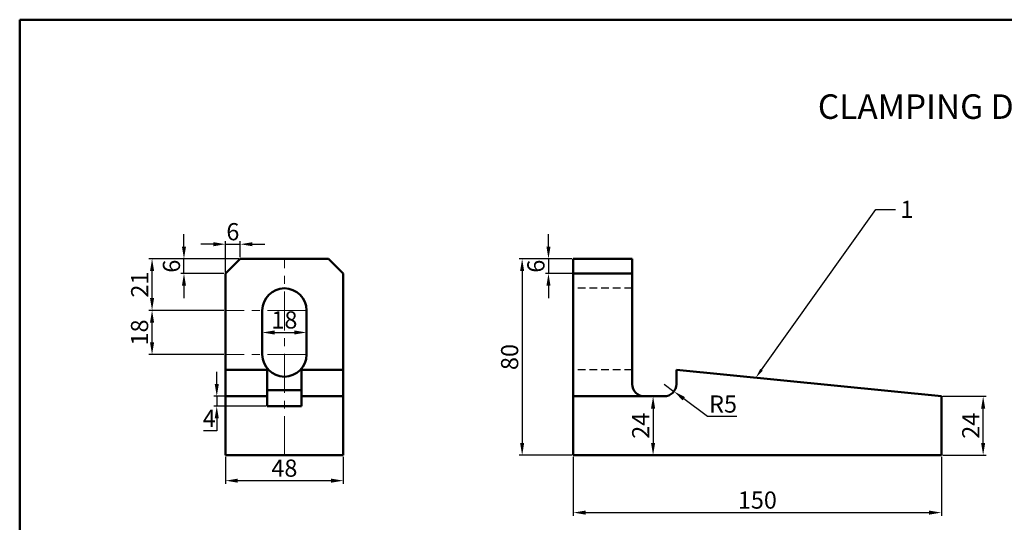
# Model space of a CAD drawing. Units: millimetres. Extents: x -238 to 500, y -191 to 322.
# Tile 2 of 3: x -238 to 164, y 117 to 322. Entities that reach past the tile are written whole.
import ezdxf
from ezdxf import colors
from ezdxf.entities.mleader import LeaderData, LeaderLine
from ezdxf.math import Vec2, Vec3

# ---------------------------------------------------------------- set-up
doc = ezdxf.new("R2010")
doc.units = ezdxf.units.MM
doc.header["$LTSCALE"] = 0.5
doc.linetypes.add('CENTER', pattern=[50.8, 31.75, -6.35, 6.35, -6.35])
doc.linetypes.add('DASHED', pattern=[19.05, 12.7, -6.35])
for name, color, linetype, lineweight in [('M-CNTR', 1, 'CENTER', 18), ('M-DIMS', 2, 'Continuous', 25), ('M-HIDN', 6, 'DASHED', 25), ('M-OUTL', 7, 'Continuous', 50), ('M-TEXT', 3, 'Continuous', 25), ('M-TTLB', 7, 'Continuous', 50)]:
    doc.layers.add(name, color=color, linetype=linetype, lineweight=lineweight)
doc.styles.get("Standard").update_dxf_attribs({"font": 'arial.ttf'})
doc.dimstyles.new('ISO-25', dxfattribs={"dimtxt": 7, "dimasz": 5, "dimexe": 1.25, "dimexo": 0.625, "dimtad": 1, "dimtoh": 1, "dimtxsty": 'Standard', "dimcen": 2.5, "dimadec": 0, "dimazin": 0, "dimtfac": 1, "dimtmove": 0, "dimatfit": 3, "dimfxl": 1, "dimarcsym": 0})

# ---------------------------------------------------------------- blocks, each defined once
blk = doc.blocks.new('*D5')
at = {"layer": 'Defpoints', "color": 0, "ltscale": 0.5, "transparency": 16777216}
for p in [(-12.02, 144.24), (137.98, 144.24), (137.98, 120.87)]:
    blk.add_point(p, dxfattribs=at)
at = {"layer": 'M-DIMS', "color": 0, "lineweight": -2, "ltscale": 0.5, "transparency": 16777216}
for p, q in [((-12.02, 143.61), (-12.02, 119.62)), ((137.98, 143.61), (137.98, 119.62)), ((-7.02, 120.87), (132.98, 120.87))]:
    blk.add_line(p, q, dxfattribs=at)
at = {"layer": 'M-DIMS', "color": 0, "ltscale": 0.5, "transparency": 16777216}
for points in [[(-7.02, 121.7), (-7.02, 120.04), (-12.02, 120.87)], [(132.98, 121.7), (132.98, 120.04), (137.98, 120.87)]]:
    blk.add_solid(points, dxfattribs=at)
at = {"layer": 'M-DIMS', "color": 0, "ltscale": 0.5, "transparency": 16777216, "insert": (62.98, 125.07), "char_height": 7, "attachment_point": 5}
blk.add_mtext('150', dxfattribs=at)
blk = doc.blocks.new('*D6')
at = {"layer": 'Defpoints', "color": 0, "ltscale": 0.5, "transparency": 16777216}
for p in [(-12.02, 224.24), (-32.87, 144.24), (-12.02, 144.24)]:
    blk.add_point(p, dxfattribs=at)
at = {"layer": 'M-DIMS', "color": 0, "lineweight": -2, "ltscale": 0.5, "transparency": 16777216}
for p, q in [((-12.65, 224.24), (-34.12, 224.24)), ((-32.87, 219.24), (-32.87, 149.24)), ((-12.65, 144.24), (-34.12, 144.24))]:
    blk.add_line(p, q, dxfattribs=at)
at = {"layer": 'M-DIMS', "color": 0, "ltscale": 0.5, "transparency": 16777216}
for points in [[(-33.71, 219.24), (-32.04, 219.24), (-32.87, 224.24)], [(-33.71, 149.24), (-32.04, 149.24), (-32.87, 144.24)]]:
    blk.add_solid(points, dxfattribs=at)
at = {"layer": 'M-DIMS', "color": 0, "ltscale": 0.5, "transparency": 16777216, "insert": (-37.07, 184.24), "char_height": 7, "attachment_point": 5, "rotation": 90}
blk.add_mtext('80', dxfattribs=at)
blk = doc.blocks.new('*D7')
at = {"layer": 'Defpoints', "color": 0, "ltscale": 0.5, "transparency": 16777216}
for p in [(-12.02, 224.24), (-22.15, 218.24), (-12.02, 218.24)]:
    blk.add_point(p, dxfattribs=at)
at = {"layer": 'M-DIMS', "color": 0, "lineweight": -2, "ltscale": 0.5, "transparency": 16777216}
for p, q in [((-22.15, 229.24), (-22.15, 234.24)), ((-12.65, 224.24), (-23.4, 224.24)), ((-22.15, 224.24), (-22.15, 218.24)), ((-12.65, 218.24), (-23.4, 218.24)), ((-22.15, 213.24), (-22.15, 208.24))]:
    blk.add_line(p, q, dxfattribs=at)
at = {"layer": 'M-DIMS', "color": 0, "ltscale": 0.5, "transparency": 16777216}
for points in [[(-22.99, 229.24), (-21.32, 229.24), (-22.15, 224.24)], [(-22.99, 213.24), (-21.32, 213.24), (-22.15, 218.24)]]:
    blk.add_solid(points, dxfattribs=at)
at = {"layer": 'M-DIMS', "color": 0, "ltscale": 0.5, "transparency": 16777216, "insert": (-26.35, 221.24), "char_height": 7, "attachment_point": 5, "rotation": 90}
blk.add_mtext('6', dxfattribs=at)
blk = doc.blocks.new('*D8')
at = {"layer": 'Defpoints', "color": 0, "ltscale": 0.5, "transparency": 16777216}
for p in [(137.98, 168.24), (155, 168.24), (137.98, 144.24)]:
    blk.add_point(p, dxfattribs=at)
at = {"layer": 'M-DIMS', "color": 0, "lineweight": -2, "ltscale": 0.5, "transparency": 16777216}
for p, q in [((138.6, 168.24), (156.25, 168.24)), ((155, 149.24), (155, 163.24)), ((138.6, 144.24), (156.25, 144.24))]:
    blk.add_line(p, q, dxfattribs=at)
at = {"layer": 'M-DIMS', "color": 0, "ltscale": 0.5, "transparency": 16777216}
for points in [[(154.16, 163.24), (155.83, 163.24), (155, 168.24)], [(154.16, 149.24), (155.83, 149.24), (155, 144.24)]]:
    blk.add_solid(points, dxfattribs=at)
at = {"layer": 'M-DIMS', "color": 0, "ltscale": 0.5, "transparency": 16777216, "insert": (150.86, 156.24), "char_height": 7, "attachment_point": 5, "rotation": 90}
blk.add_mtext('24', dxfattribs=at)
blk = doc.blocks.new('*D9')
at = {"layer": 'Defpoints', "color": 0, "ltscale": 0.5, "transparency": 16777216}
for p in [(20.98, 168.24), (20.49, 144.24), (20.98, 144.24)]:
    blk.add_point(p, dxfattribs=at)
at = {"layer": 'M-DIMS', "color": 0, "lineweight": -2, "ltscale": 0.5, "transparency": 16777216}
for p, q in [((20.35, 168.24), (19.24, 168.24)), ((20.49, 163.24), (20.49, 149.24)), ((20.35, 144.24), (19.24, 144.24))]:
    blk.add_line(p, q, dxfattribs=at)
at = {"layer": 'M-DIMS', "color": 0, "ltscale": 0.5, "transparency": 16777216}
for points in [[(19.65, 163.24), (21.32, 163.24), (20.49, 168.24)], [(19.65, 149.24), (21.32, 149.24), (20.49, 144.24)]]:
    blk.add_solid(points, dxfattribs=at)
at = {"layer": 'M-DIMS', "color": 0, "ltscale": 0.5, "transparency": 16777216, "insert": (16.35, 156.24), "char_height": 7, "attachment_point": 5, "rotation": 90}
blk.add_mtext('24', dxfattribs=at)
blk = doc.blocks.new('*D10')
at = {"layer": 'Defpoints', "color": 0, "ltscale": 0.5, "transparency": 16777216}
for p in [(24.98, 173.24), (28.98, 170.25)]:
    blk.add_point(p, dxfattribs=at)
at = {"layer": 'M-DIMS', "color": 0, "lineweight": -2, "ltscale": 0.5, "transparency": 16777216}
for p, q in [((24.98, 173.24), (28.98, 170.25)), ((42.7, 160.01), (32.99, 167.26)), ((54.67, 160.01), (42.7, 160.01))]:
    blk.add_line(p, q, dxfattribs=at)
at = {"layer": 'M-DIMS', "color": 0, "ltscale": 0.5, "transparency": 16777216}
blk.add_solid([(33.49, 167.92), (32.49, 166.59), (28.98, 170.25)], dxfattribs=at)
at = {"layer": 'M-DIMS', "color": 0, "ltscale": 0.5, "transparency": 16777216, "insert": (49, 164.19), "char_height": 7, "attachment_point": 5}
blk.add_mtext('R5', dxfattribs=at)
blk = doc.blocks.new('*D11')
at = {"layer": 'Defpoints', "color": 0, "ltscale": 0.5, "transparency": 16777216}
for p in [(-147.77, 230.19), (-147.77, 224.24), (-153.77, 218.24)]:
    blk.add_point(p, dxfattribs=at)
at = {"layer": 'M-DIMS', "color": 0, "lineweight": -2, "ltscale": 0.5, "transparency": 16777216}
for p, q in [((-158.77, 230.19), (-163.77, 230.19)), ((-153.77, 218.86), (-153.77, 231.44)), ((-153.77, 230.19), (-147.77, 230.19)), ((-147.77, 224.86), (-147.77, 231.44)), ((-142.77, 230.19), (-137.77, 230.19))]:
    blk.add_line(p, q, dxfattribs=at)
at = {"layer": 'M-DIMS', "color": 0, "ltscale": 0.5, "transparency": 16777216}
for points in [[(-158.77, 231.02), (-158.77, 229.35), (-153.77, 230.19)], [(-142.77, 231.02), (-142.77, 229.35), (-147.77, 230.19)]]:
    blk.add_solid(points, dxfattribs=at)
at = {"layer": 'M-DIMS', "color": 0, "ltscale": 0.5, "transparency": 16777216, "insert": (-150.77, 234.38), "char_height": 7, "attachment_point": 5}
blk.add_mtext('6', dxfattribs=at)
blk = doc.blocks.new('*D12')
at = {"layer": 'Defpoints', "color": 0, "ltscale": 0.5, "transparency": 16777216}
for p in [(-170.69, 224.24), (-147.77, 224.24), (-153.77, 218.24)]:
    blk.add_point(p, dxfattribs=at)
at = {"layer": 'M-DIMS', "color": 0, "lineweight": -2, "ltscale": 0.5, "transparency": 16777216}
for p, q in [((-170.69, 229.24), (-170.69, 234.24)), ((-148.39, 224.24), (-171.94, 224.24)), ((-170.69, 218.24), (-170.69, 224.24)), ((-154.39, 218.24), (-171.94, 218.24)), ((-170.69, 213.24), (-170.69, 208.24))]:
    blk.add_line(p, q, dxfattribs=at)
at = {"layer": 'M-DIMS', "color": 0, "ltscale": 0.5, "transparency": 16777216}
for points in [[(-171.52, 229.24), (-169.85, 229.24), (-170.69, 224.24)], [(-171.52, 213.24), (-169.85, 213.24), (-170.69, 218.24)]]:
    blk.add_solid(points, dxfattribs=at)
at = {"layer": 'M-DIMS', "color": 0, "ltscale": 0.5, "transparency": 16777216, "insert": (-174.88, 221.24), "char_height": 7, "attachment_point": 5, "rotation": 90}
blk.add_mtext('6', dxfattribs=at)
blk = doc.blocks.new('*D13')
at = {"layer": 'Defpoints', "color": 0, "ltscale": 0.5, "transparency": 16777216}
for p in [(-183.7, 224.24), (-153.77, 224.24), (-153.77, 203.24)]:
    blk.add_point(p, dxfattribs=at)
at = {"layer": 'M-DIMS', "color": 0, "lineweight": -2, "ltscale": 0.5, "transparency": 16777216}
for p, q in [((-154.39, 224.24), (-184.95, 224.24)), ((-183.7, 208.24), (-183.7, 219.24)), ((-154.39, 203.24), (-184.95, 203.24))]:
    blk.add_line(p, q, dxfattribs=at)
at = {"layer": 'M-DIMS', "color": 0, "ltscale": 0.5, "transparency": 16777216}
for points in [[(-184.53, 219.24), (-182.86, 219.24), (-183.7, 224.24)], [(-184.53, 208.24), (-182.86, 208.24), (-183.7, 203.24)]]:
    blk.add_solid(points, dxfattribs=at)
at = {"layer": 'M-DIMS', "color": 0, "ltscale": 0.5, "transparency": 16777216, "insert": (-187.83, 213.74), "char_height": 7, "attachment_point": 5, "rotation": 90}
blk.add_mtext('21', dxfattribs=at)
blk = doc.blocks.new('*D14')
at = {"layer": 'Defpoints', "color": 0, "ltscale": 0.5, "transparency": 16777216}
for p in [(-183.7, 203.24), (-153.77, 203.24), (-153.77, 185.24)]:
    blk.add_point(p, dxfattribs=at)
at = {"layer": 'M-DIMS', "color": 0, "lineweight": -2, "ltscale": 0.5, "transparency": 16777216}
for p, q in [((-154.39, 203.24), (-184.95, 203.24)), ((-183.7, 190.24), (-183.7, 198.24)), ((-154.39, 185.24), (-184.95, 185.24))]:
    blk.add_line(p, q, dxfattribs=at)
at = {"layer": 'M-DIMS', "color": 0, "ltscale": 0.5, "transparency": 16777216}
for points in [[(-184.53, 198.24), (-182.86, 198.24), (-183.7, 203.24)], [(-184.53, 190.24), (-182.86, 190.24), (-183.7, 185.24)]]:
    blk.add_solid(points, dxfattribs=at)
at = {"layer": 'M-DIMS', "color": 0, "ltscale": 0.5, "transparency": 16777216, "insert": (-187.89, 194.24), "char_height": 7, "attachment_point": 5, "rotation": 90}
blk.add_mtext('18', dxfattribs=at)
blk = doc.blocks.new('*D15')
at = {"layer": 'Defpoints', "color": 0, "ltscale": 0.5, "transparency": 16777216}
for p in [(-136.77, 168.24), (-157.33, 164.24), (-136.77, 164.24)]:
    blk.add_point(p, dxfattribs=at)
at = {"layer": 'M-DIMS', "color": 0, "lineweight": -2, "ltscale": 0.5, "transparency": 16777216}
for p, q in [((-157.33, 173.24), (-157.33, 178.24)), ((-137.39, 168.24), (-158.58, 168.24)), ((-157.33, 168.24), (-157.33, 164.24)), ((-137.39, 164.24), (-158.58, 164.24)), ((-157.33, 159.24), (-157.33, 154.24)), ((-157.33, 154.24), (-162.8, 154.24))]:
    blk.add_line(p, q, dxfattribs=at)
at = {"layer": 'M-DIMS', "color": 0, "ltscale": 0.5, "transparency": 16777216}
for points in [[(-158.17, 173.24), (-156.5, 173.24), (-157.33, 168.24)], [(-158.17, 159.24), (-156.5, 159.24), (-157.33, 164.24)]]:
    blk.add_solid(points, dxfattribs=at)
at = {"layer": 'M-DIMS', "color": 0, "ltscale": 0.5, "transparency": 16777216, "insert": (-160.38, 158.36), "char_height": 7, "attachment_point": 5}
blk.add_mtext('4', dxfattribs=at)
blk = doc.blocks.new('*D16')
at = {"layer": 'Defpoints', "color": 0, "ltscale": 0.5, "transparency": 16777216}
for p in [(-153.77, 144.24), (-105.77, 144.24), (-105.77, 133.88)]:
    blk.add_point(p, dxfattribs=at)
at = {"layer": 'M-DIMS', "color": 0, "lineweight": -2, "ltscale": 0.5, "transparency": 16777216}
for p, q in [((-153.77, 143.61), (-153.77, 132.63)), ((-105.77, 143.61), (-105.77, 132.63)), ((-148.77, 133.88), (-110.77, 133.88))]:
    blk.add_line(p, q, dxfattribs=at)
at = {"layer": 'M-DIMS', "color": 0, "ltscale": 0.5, "transparency": 16777216}
for points in [[(-148.77, 134.71), (-148.77, 133.05), (-153.77, 133.88)], [(-110.77, 134.71), (-110.77, 133.05), (-105.77, 133.88)]]:
    blk.add_solid(points, dxfattribs=at)
at = {"layer": 'M-DIMS', "color": 0, "ltscale": 0.5, "transparency": 16777216, "insert": (-129.77, 138.08), "char_height": 7, "attachment_point": 5}
blk.add_mtext('48', dxfattribs=at)
blk = doc.blocks.new('*D17')
at = {"layer": 'Defpoints', "color": 0, "ltscale": 0.5, "transparency": 16777216}
for p in [(-138.77, 194.24), (-120.77, 194.24), (-120.77, 194.24)]:
    blk.add_point(p, dxfattribs=at)
at = {"layer": 'M-DIMS', "color": 0, "lineweight": -2, "ltscale": 0.5, "transparency": 16777216}
for p, q in [((-138.77, 194.86), (-138.77, 195.49)), ((-133.77, 194.24), (-125.77, 194.24)), ((-120.77, 194.86), (-120.77, 195.49))]:
    blk.add_line(p, q, dxfattribs=at)
at = {"layer": 'M-DIMS', "color": 0, "ltscale": 0.5, "transparency": 16777216}
for points in [[(-133.77, 195.07), (-133.77, 193.4), (-138.77, 194.24)], [(-125.77, 195.07), (-125.77, 193.4), (-120.77, 194.24)]]:
    blk.add_solid(points, dxfattribs=at)
at = {"layer": 'M-DIMS', "color": 0, "ltscale": 0.5, "transparency": 16777216, "insert": (-129.77, 198.44), "char_height": 7, "attachment_point": 5}
blk.add_mtext('18', dxfattribs=at)

msp = doc.modelspace()

# ---------------------------------------------------------------- linework, layer by layer
at = {"layer": 'M-CNTR'}
for p, q in [((-129.768, 144.238), (-129.768, 224.238)), ((-120.768, 203.238), (-153.768, 203.238)), ((-120.768, 185.238), (-153.768, 185.238))]:
    msp.add_line(p, q, dxfattribs=at)
at = {"layer": 'M-HIDN', "ltscale": 0.5}
for p, q in [((11.976, 212.238), (-12.024, 212.238)), ((11.976, 179.037), (-12.024, 179.037))]:
    msp.add_line(p, q, dxfattribs=at)
at = {"layer": 'M-OUTL', "ltscale": 0.5}
for p, q in [((-153.768, 218.238), (-147.768, 224.238)), ((-105.768, 218.238), (-111.768, 224.238))]:
    msp.add_line(p, q, dxfattribs=at)
at = {"layer": 'M-OUTL'}
for p, q in [((-111.768, 224.238), (-147.768, 224.238)), ((-12.024, 224.238), (-12.024, 144.238)), ((-12.024, 224.238), (11.976, 224.238)), ((11.976, 224.238), (11.976, 173.238)), ((-153.768, 218.238), (-153.768, 144.238)), ((-105.768, 144.238), (-105.768, 218.238)), ((-12.024, 218.238), (11.976, 218.238)), ((-138.768, 203.238), (-138.768, 185.238)), ((-120.768, 203.238), (-120.768, 185.238)), ((-136.768, 164.238), (-136.768, 179.037)), ((-122.768, 164.238), (-122.768, 179.037)), ((137.976, 168.238), (29.976, 179.037)), ((29.976, 179.037), (29.976, 173.238)), ((-122.768, 170.738), (-136.768, 170.738)), ((-136.768, 168.238), (-153.768, 168.238)), ((-105.768, 168.238), (-122.768, 168.238)), ((16.976, 168.238), (-12.024, 168.238)), ((16.976, 168.238), (24.976, 168.238)), ((137.976, 144.238), (137.976, 168.238)), ((-122.768, 164.238), (-136.768, 164.238)), ((-153.768, 144.238), (-105.768, 144.238)), ((-12.024, 144.238), (137.976, 144.238))]:
    msp.add_line(p, q, dxfattribs=at)
for points in [[(-136.768, 179.037), (-153.768, 179.037)], [(-105.768, 179.037), (-122.768, 179.037)]]:
    msp.add_lwpolyline(points, dxfattribs=at)
for centre, radius, start, end in [((-129.768, 203.238), 9, 0, 180), ((-129.768, 185.238), 9, 180, 0), ((16.976, 173.238), 5, 180, 270), ((24.976, 173.238), 5, 270, 0)]:
    msp.add_arc(centre, radius, start, end, dxfattribs=at)
at = {"layer": 'M-TTLB', "ltscale": 0.5}
msp.add_lwpolyline([(-237.643, 321.636), (499.641, 321.636), (499.641, -152.379), (-237.643, -152.379)], close=True, dxfattribs=at)

# ---------------------------------------------------------------- texts
at = {"layer": 'M-TEXT', "ltscale": 0.5, "insert": (87.633, 291.237), "char_height": 10, "attachment_point": 1}
msp.add_mtext_dynamic_manual_height_columns('CLAMPING DEVICE', width=136.41378, gutter_width=12.5, heights=[0], dxfattribs=at)

# ---------------------------------------------------------------- dimensions: what is measured, and where the dimension line sits
at = {"layer": 'M-DIMS', "ltscale": 0.5}
for base, p1, p2, picture, middle in [((-147.768, 230.185), (-153.768, 218.238), (-147.768, 224.238), '*D11', (-150.768, 234.384)), ((-120.768, 194.238), (-138.768, 194.238), (-120.768, 194.238), '*D17', (-129.768, 198.437)), ((-105.768, 133.881), (-153.768, 144.238), (-105.768, 144.238), '*D16', (-129.768, 138.08)), ((137.976, 120.872), (-12.024, 144.238), (137.976, 144.238), '*D5', (62.976, 125.071))]:
    dim = msp.add_linear_dim(base=base, p1=p1, p2=p2, dimstyle='ISO-25', override={"dimclrd": 0, "dimclre": 0, "dimclrt": 0}, dxfattribs=at)
    dim.commit()
    dim.dimension.update_dxf_attribs({"geometry": picture, "text_midpoint": middle})
for base, p1, p2, picture, middle in [((-170.686, 224.238), (-153.768, 218.238), (-147.768, 224.238), '*D12', (-170.686, 221.238)), ((-183.695, 203.238), (-153.768, 185.238), (-153.768, 203.238), '*D14', (-183.695, 194.238))]:
    dim = msp.add_linear_dim(base=base, p1=p1, p2=p2, angle=90, dimstyle='ISO-25', override={"dimclrd": 0, "dimclre": 0, "dimclrt": 0}, dxfattribs=at)
    dim.commit()
    dim.dimension.update_dxf_attribs({"geometry": picture, "text_midpoint": middle, "dimtype": 160})
for base, p1, p2, picture, middle in [((-22.152, 218.238), (-12.024, 224.238), (-12.024, 218.238), '*D7', (-26.351, 221.238)), ((-183.695, 224.238), (-153.768, 203.238), (-153.768, 224.238), '*D13', (-187.835, 213.738)), ((-32.873, 144.238), (-12.024, 224.238), (-12.024, 144.238), '*D6', (-37.072, 184.238)), ((-157.334, 164.238), (-136.768, 168.238), (-136.768, 164.238), '*D15', (-160.38, 158.363)), ((20.486, 144.238), (20.976, 168.238), (20.976, 144.238), '*D9', (16.347, 156.238)), ((154.997, 168.238), (137.976, 144.238), (137.976, 168.238), '*D8', (150.858, 156.238))]:
    dim = msp.add_linear_dim(base=base, p1=p1, p2=p2, angle=90, dimstyle='ISO-25', override={"dimclrd": 0, "dimclre": 0, "dimclrt": 0}, dxfattribs=at)
    dim.commit()
    dim.dimension.update_dxf_attribs({"geometry": picture, "text_midpoint": middle})
dim = msp.add_radius_dim(center=(24.976, 173.238), mpoint=(28.983, 170.247), dimstyle='ISO-25', override={"dimclrd": 0, "dimclre": 0, "dimclrt": 0}, dxfattribs=at)
dim.commit()
dim.dimension.update_dxf_attribs({"geometry": '*D10', "text_midpoint": (48.996, 164.19)})

# ---------------------------------------------------------------- leaders
at = {"layer": 'M-TEXT', "ltscale": 0.5}
ml = msp.add_multileader_mtext('Standard', dxfattribs=at)
ml.set_content('1', color=256)
ml.set_leader_properties()
ml.build(insert=Vec2(0, 0))
ctx = ml.context
ctx.base_point, ctx.char_height, ctx.plane_origin = Vec3(119.283, 244.391), 7, Vec3(62.352, 175.8)
notes = []
notes.append((ctx, [(0, (1, 1, 0), (111.283, 244.391), (1, 0), 8, [(0, [(62.352, 175.8)], 0, [])])]))
ctx.mtext.insert, ctx.mtext.flow_direction = Vec3(121.283, 247.891), 5
for ctx, leaders in notes:
    for number, flags, end, landing, length, lines in leaders:
        leader = LeaderData()
        leader.index, (leader.has_last_leader_line, leader.has_dogleg_vector, leader.attachment_direction) = number, flags
        leader.last_leader_point, leader.dogleg_vector, leader.dogleg_length = Vec3(end), Vec3(landing), length
        for number, points, colour, breaks in lines:
            line = LeaderLine()
            line.index, line.vertices, line.color, line.breaks = number, Vec3.list(points), colors.encode_raw_color(colour), breaks
            leader.lines.append(line)
        ctx.leaders.append(leader)

doc.saveas('drawing.dxf')
